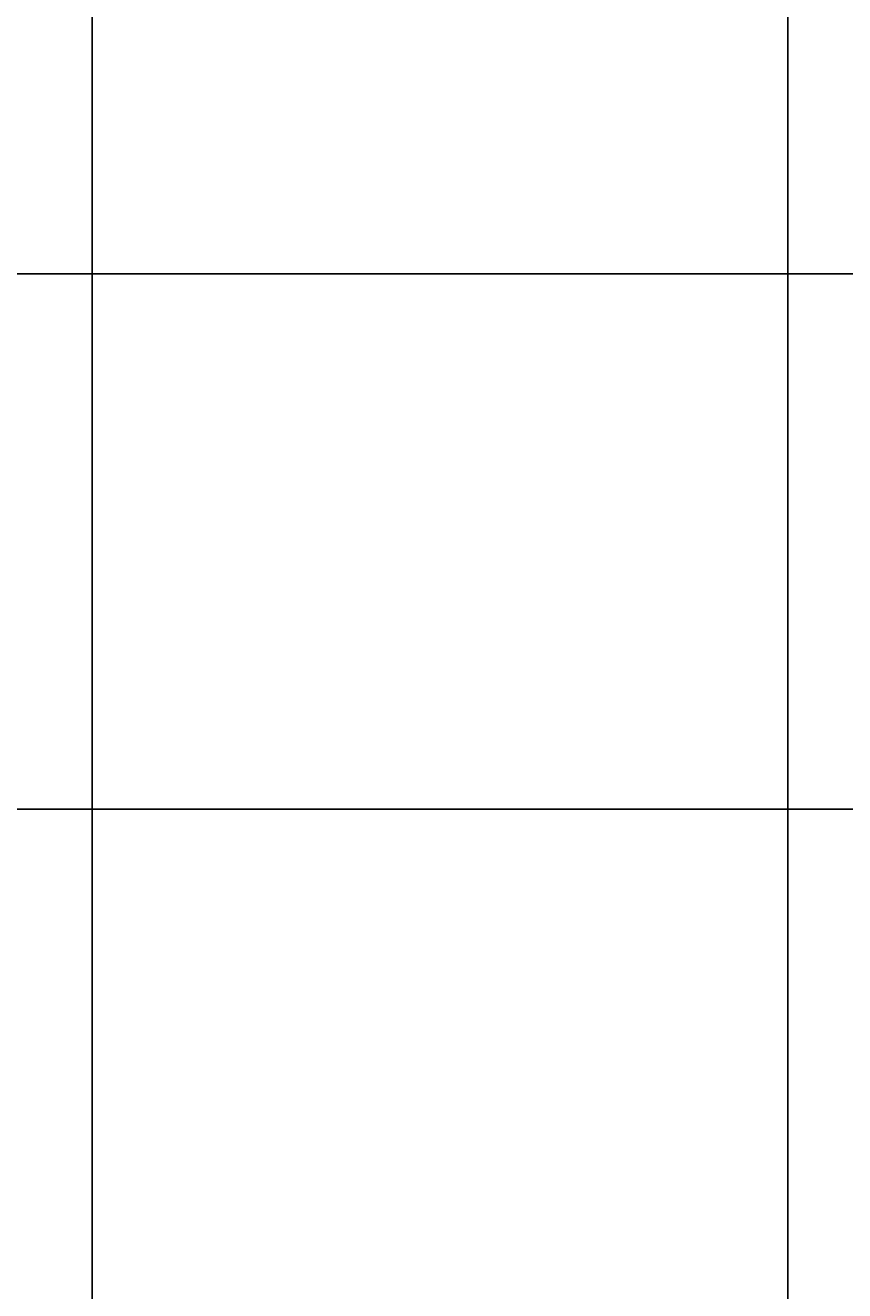
# Model space of a CAD drawing. Units: feet. Extents: x 105 to 1094, y -88 to 588.
# Tile 51 of 59: x 551 to 575, y 513 to 551. Entities that reach past the tile are written whole.
import ezdxf

# ---------------------------------------------------------------- set-up
doc = ezdxf.new("R2010")
doc.units = ezdxf.units.FT
doc.header["$MEASUREMENT"] = 0
doc.layers.add('A-ANNO-DIMS', color=2, linetype='Continuous', lineweight=18)
doc.styles.get("Standard").update_dxf_attribs({"font": 'arial.ttf'})
doc.dimstyles.get("Standard").update_dxf_attribs({"dimtxt": 0.18, "dimasz": 0.18, "dimexe": 0.18, "dimexo": 0.0625, "dimgap": 0.09, "dimtad": 0, "dimtih": 1, "dimtoh": 1, "dimdec": 4, "dimzin": 0, "dimdsep": 46, "dimtxsty": 'Standard', "dimcen": 0.09, "dimadec": 0, "dimazin": 0, "dimtfac": 1, "dimtdec": 4, "dimtofl": 0, "dimtmove": 0, "dimatfit": 3, "dimfxl": 1, "dimtolj": 1, "dimtzin": 0, "dimarcsym": 0})

# ---------------------------------------------------------------- blocks, each defined once
blk = doc.blocks.new('*D21')
at = {"layer": 'A-ANNO-DIMS', "color": 0, "lineweight": -2, "transparency": 16777216}
for p, q in [((849.626, 543.081), (105.458, 543.081)), ((105.638, 542.901), (105.638, 250.263)), ((105.638, -42.739), (105.638, 249.899)), ((849.626, -42.919), (105.458, -42.919))]:
    blk.add_line(p, q, dxfattribs=at)
at = {"layer": 'A-ANNO-DIMS', "color": 0, "transparency": 16777216}
for points in [[(105.608, 542.901), (105.668, 542.901), (105.638, 543.081)], [(105.608, -42.739), (105.668, -42.739), (105.638, -42.919)]]:
    blk.add_solid(points, dxfattribs=at)
at = {"layer": 'Defpoints', "color": 0, "transparency": 16777216}
for p in [(105.638, 543.081), (849.688, 543.081), (849.688, -42.919)]:
    blk.add_point(p, dxfattribs=at)
at = {"layer": 'A-ANNO-DIMS', "color": 0, "transparency": 16777216, "insert": (105.638, 250.081), "char_height": 0.18, "attachment_point": 5}
blk.add_mtext('\\A1;586', dxfattribs=at)
blk = doc.blocks.new('*D25')
at = {"layer": 'A-ANNO-DIMS', "color": 0, "lineweight": -2, "transparency": 16777216}
for p, q in [((438.688, 527.144), (438.688, 588.311)), ((552.688, 471.144), (552.688, 588.311)), ((438.868, 588.131), (495.408, 588.131)), ((552.508, 588.131), (495.968, 588.131))]:
    blk.add_line(p, q, dxfattribs=at)
at = {"layer": 'A-ANNO-DIMS', "color": 0, "transparency": 16777216}
for points in [[(438.868, 588.161), (438.868, 588.101), (438.688, 588.131)], [(552.508, 588.161), (552.508, 588.101), (552.688, 588.131)]]:
    blk.add_solid(points, dxfattribs=at)
at = {"layer": 'Defpoints', "color": 0, "transparency": 16777216}
for p in [(552.688, 588.131), (438.688, 527.081), (552.688, 471.081)]:
    blk.add_point(p, dxfattribs=at)
at = {"layer": 'A-ANNO-DIMS', "color": 0, "transparency": 16777216, "insert": (495.688, 588.131), "char_height": 0.18, "attachment_point": 5}
blk.add_mtext('\\A1;114', dxfattribs=at)
blk = doc.blocks.new('*D26')
at = {"layer": 'A-ANNO-DIMS', "color": 0, "lineweight": -2, "transparency": 16777216}
for p, q in [((552.688, 471.144), (552.688, 588.311)), ((646.688, 471.144), (646.688, 588.311)), ((552.868, 588.131), (599.47, 588.131)), ((646.508, 588.131), (599.907, 588.131))]:
    blk.add_line(p, q, dxfattribs=at)
at = {"layer": 'A-ANNO-DIMS', "color": 0, "transparency": 16777216}
for points in [[(552.868, 588.161), (552.868, 588.101), (552.688, 588.131)], [(646.508, 588.161), (646.508, 588.101), (646.688, 588.131)]]:
    blk.add_solid(points, dxfattribs=at)
at = {"layer": 'Defpoints', "color": 0, "transparency": 16777216}
for p in [(646.688, 588.131), (552.688, 471.081), (646.688, 471.081)]:
    blk.add_point(p, dxfattribs=at)
at = {"layer": 'A-ANNO-DIMS', "color": 0, "transparency": 16777216, "insert": (599.688, 588.131), "char_height": 0.18, "attachment_point": 5}
blk.add_mtext('\\A1;94', dxfattribs=at)
blk = doc.blocks.new('*D30')
at = {"layer": 'A-ANNO-DIMS', "color": 0, "lineweight": -2, "transparency": 16777216}
for p, q in [((349.751, 543.081), (1093.918, 543.081)), ((1093.738, 542.901), (1093.738, 535.263)), ((1093.738, 527.261), (1093.738, 534.899)), ((349.751, 527.081), (1093.918, 527.081))]:
    blk.add_line(p, q, dxfattribs=at)
at = {"layer": 'A-ANNO-DIMS', "color": 0, "transparency": 16777216}
for points in [[(1093.708, 542.901), (1093.768, 542.901), (1093.738, 543.081)], [(1093.708, 527.261), (1093.768, 527.261), (1093.738, 527.081)]]:
    blk.add_solid(points, dxfattribs=at)
at = {"layer": 'Defpoints', "color": 0, "transparency": 16777216}
for p in [(349.688, 543.081), (349.688, 527.081), (1093.738, 527.081)]:
    blk.add_point(p, dxfattribs=at)
at = {"layer": 'A-ANNO-DIMS', "color": 0, "transparency": 16777216, "insert": (1093.738, 535.081), "char_height": 0.18, "attachment_point": 5}
blk.add_mtext('\\A1;16', dxfattribs=at)
blk = doc.blocks.new('*D31')
at = {"layer": 'A-ANNO-DIMS', "color": 0, "lineweight": -2, "transparency": 16777216}
for p, q in [((438.751, 527.081), (1093.918, 527.081)), ((1093.738, 526.901), (1093.738, 499.263)), ((1093.738, 471.261), (1093.738, 498.899)), ((438.751, 471.081), (1093.918, 471.081))]:
    blk.add_line(p, q, dxfattribs=at)
at = {"layer": 'A-ANNO-DIMS', "color": 0, "transparency": 16777216}
for points in [[(1093.708, 526.901), (1093.768, 526.901), (1093.738, 527.081)], [(1093.708, 471.261), (1093.768, 471.261), (1093.738, 471.081)]]:
    blk.add_solid(points, dxfattribs=at)
at = {"layer": 'Defpoints', "color": 0, "transparency": 16777216}
for p in [(438.688, 527.081), (1093.738, 527.081), (438.688, 471.081)]:
    blk.add_point(p, dxfattribs=at)
at = {"layer": 'A-ANNO-DIMS', "color": 0, "transparency": 16777216, "insert": (1093.738, 499.081), "char_height": 0.18, "attachment_point": 5}
blk.add_mtext('\\A1;56', dxfattribs=at)
blk = doc.blocks.new('*D47')
at = {"layer": 'A-ANNO-DIMS', "color": 0, "lineweight": -2, "transparency": 16777216}
for p, q in [((552.688, 441.144), (552.688, 588.311)), ((573.483, 441.144), (573.483, 588.311)), ((552.868, 588.131), (562.621, 588.131)), ((573.303, 588.131), (563.55, 588.131))]:
    blk.add_line(p, q, dxfattribs=at)
at = {"layer": 'A-ANNO-DIMS', "color": 0, "transparency": 16777216}
for points in [[(552.868, 588.161), (552.868, 588.101), (552.688, 588.131)], [(573.303, 588.161), (573.303, 588.101), (573.483, 588.131)]]:
    blk.add_solid(points, dxfattribs=at)
at = {"layer": 'Defpoints', "color": 0, "transparency": 16777216}
for p in [(573.483, 588.131), (552.688, 441.081), (573.483, 441.081)]:
    blk.add_point(p, dxfattribs=at)
at = {"layer": 'A-ANNO-DIMS', "color": 0, "transparency": 16777216, "insert": (563.085, 588.131), "char_height": 0.18, "attachment_point": 5}
blk.add_mtext('\\A1;20.794', dxfattribs=at)
blk = doc.blocks.new('*D48')
at = {"layer": 'A-ANNO-DIMS', "color": 0, "lineweight": -2, "transparency": 16777216}
for p, q in [((573.483, 441.144), (573.483, 588.311)), ((633.483, 441.144), (633.483, 588.311)), ((573.663, 588.131), (603.263, 588.131)), ((633.303, 588.131), (603.702, 588.131))]:
    blk.add_line(p, q, dxfattribs=at)
at = {"layer": 'A-ANNO-DIMS', "color": 0, "transparency": 16777216}
for points in [[(573.663, 588.161), (573.663, 588.101), (573.483, 588.131)], [(633.303, 588.161), (633.303, 588.101), (633.483, 588.131)]]:
    blk.add_solid(points, dxfattribs=at)
at = {"layer": 'Defpoints', "color": 0, "transparency": 16777216}
for p in [(633.483, 588.131), (573.483, 441.081), (633.483, 441.081)]:
    blk.add_point(p, dxfattribs=at)
at = {"layer": 'A-ANNO-DIMS', "color": 0, "transparency": 16777216, "insert": (603.483, 588.131), "char_height": 0.18, "attachment_point": 5}
blk.add_mtext('\\A1;60', dxfattribs=at)

msp = doc.modelspace()

# ---------------------------------------------------------------- dimensions: what is measured, and where the dimension line sits
at = {"layer": 'A-ANNO-DIMS'}
for base, p1, p2, override, picture, middle in [((552.6883, 588.1312), (438.6883, 527.0812), (552.6883, 471.0812), {"dimdec": 0, "dimlfac": 1, "dimrnd": 0, "dimzin": 0, "dimdsep": 46, "dimlunit": 2}, '*D25', (495.6883, 588.1312)), ((646.6883, 588.1312), (552.6883, 471.0812), (646.6883, 471.0812), {"dimdec": 0, "dimlfac": 1, "dimrnd": 0, "dimzin": 0, "dimdsep": 46, "dimlunit": 2}, '*D26', (599.6883, 588.1312)), ((573.4826, 588.1312), (552.6883, 441.0812), (573.4826, 441.0812), {"dimdec": 3, "dimlfac": 1, "dimrnd": 0, "dimzin": 0, "dimdsep": 46, "dimlunit": 2}, '*D47', (563.0854, 588.1312)), ((633.4826, 588.1312), (573.4826, 441.0812), (633.4826, 441.0812), {"dimdec": 0, "dimlfac": 1, "dimrnd": 0, "dimzin": 0, "dimdsep": 46, "dimlunit": 2}, '*D48', (603.4826, 588.1312))]:
    dim = msp.add_linear_dim(base=base, p1=p1, p2=p2, dimstyle='Standard', override=override, dxfattribs=at)
    dim.commit()
    dim.dimension.update_dxf_attribs({"geometry": picture, "text_midpoint": middle})
for base, p1, p2, picture, middle in [((105.6383, 543.0812), (849.6883, -42.9188), (849.6883, 543.0812), '*D21', (105.6383, 250.0812)), ((1093.7383, 527.0812), (349.6883, 543.0812), (349.6883, 527.0812), '*D30', (1093.7383, 535.0812)), ((1093.7383, 527.0812), (438.6883, 471.0812), (438.6883, 527.0812), '*D31', (1093.7383, 499.0812))]:
    dim = msp.add_linear_dim(base=base, p1=p1, p2=p2, angle=90, dimstyle='Standard', override={"dimdec": 0, "dimlfac": 1, "dimrnd": 0, "dimzin": 0, "dimdsep": 46, "dimlunit": 2}, dxfattribs=at)
    dim.commit()
    dim.dimension.update_dxf_attribs({"geometry": picture, "text_midpoint": middle})

doc.saveas('drawing.dxf')
